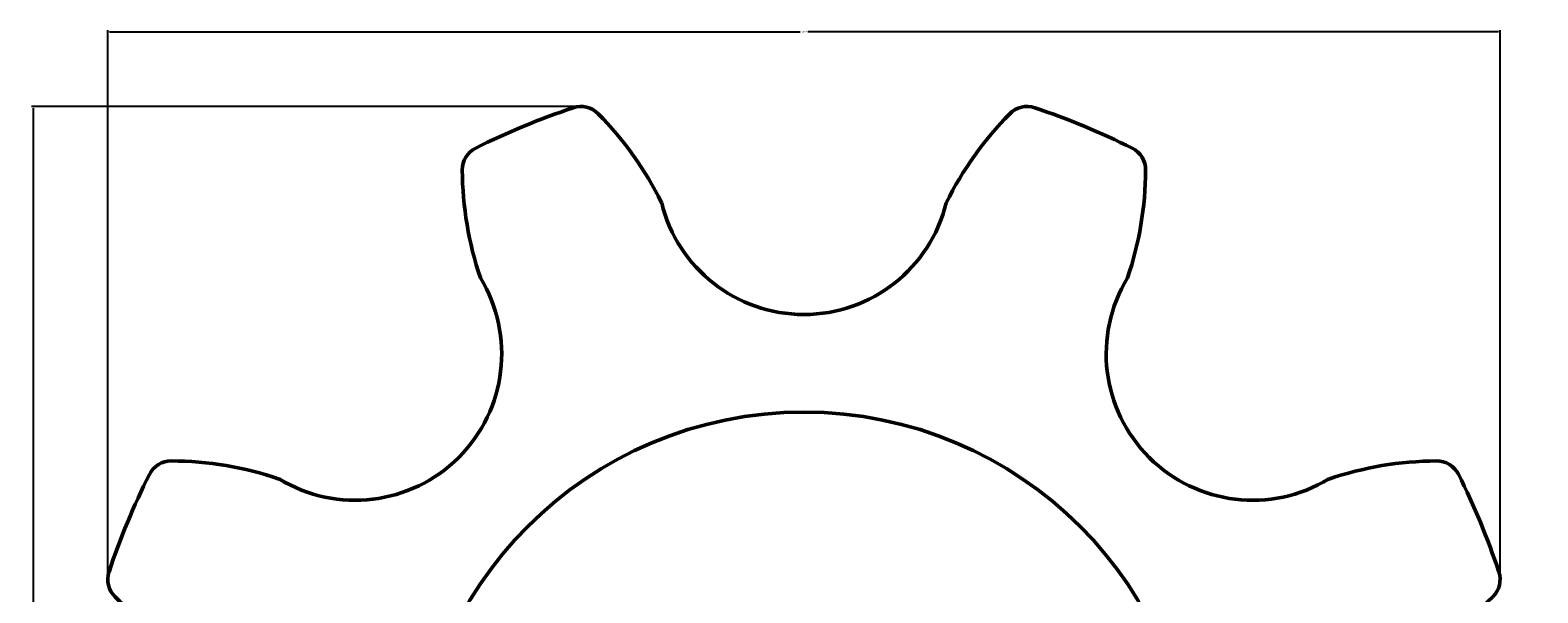
# Model space of a CAD drawing. Units: millimetres. Extents: x 7298 to 7452, y 8725 to 8883.
# Tile 2 of 2: x 7298 to 7452, y 8826 to 8883. Entities that reach past the tile are written whole.
import ezdxf

# ---------------------------------------------------------------- set-up
doc = ezdxf.new("R2010")
doc.units = ezdxf.units.MM
doc.layers.add('M-DIMS', color=2, linetype='Continuous', lineweight=18)
doc.layers.add('M-OUTL', color=7, linetype='Continuous', lineweight=50)
doc.styles.get("Standard").update_dxf_attribs({"font": 'arial.ttf'})
doc.dimstyles.get("Standard").update_dxf_attribs({"dimtxt": 0.18, "dimasz": 0.18, "dimexe": 0.18, "dimexo": 0.0625, "dimgap": 0.09, "dimtad": 0, "dimtih": 1, "dimtoh": 1, "dimdec": 4, "dimzin": 0, "dimdsep": 46, "dimtxsty": 'Standard', "dimcen": 0.09, "dimadec": 0, "dimazin": 0, "dimtfac": 1, "dimtdec": 4, "dimtofl": 0, "dimtmove": 0, "dimatfit": 3, "dimfxl": 1, "dimtolj": 1, "dimtzin": 0, "dimarcsym": 0})

# ---------------------------------------------------------------- blocks, each defined once
blk = doc.blocks.new('*U1')
for centre, radius, start, end in [((-2.28, 7.71), 2.5, 89.661, 153.3674), ((-2.47, -24.79), 35, 71.2539, 89.661), ((62.53, -24.79), 75, 153.3674, 161.6326), ((-6.28, -1.94), 2.5, 161.6326, 225.339), ((16.57, 21.18), 35, 225.339, 243.7461)]:
    blk.add_arc(centre, radius, start, end)
blk = doc.blocks.new('*U2')
at = {"layer": 'M-OUTL', "color": 0, "linetype": 'ByBlock', "lineweight": -2, "transparency": 16777216}
for p, rotation in [((7350.2, 8866.09), 315.0000000000001), ((7401.68, 8866.87), 270), ((7438.63, 8831.03), 225), ((7315.15, 8777.66), 44.99999999999996), ((7439.42, 8779.56), 180), ((7403.58, 8742.6), 134.9999999999999), ((7352.11, 8741.82), 90)]:
    blk.add_blockref('*U1', p, dxfattribs=dict(at, rotation=rotation))
blk.add_blockref('*U1', (7314.36, 8829.13), dxfattribs=at)
blk = doc.blocks.new('*D3')
at = {"layer": 'Defpoints', "color": 0, "transparency": 16777216}
for p in [(7448.2, 8883.3), (7305.59, 8827.29), (7448.2, 8827.29)]:
    blk.add_point(p, dxfattribs=at)
at = {"layer": 'M-DIMS', "color": 0, "lineweight": -2, "transparency": 16777216}
for p, q in [((7305.59, 8827.35), (7305.59, 8883.48)), ((7305.77, 8883.3), (7376.51, 8883.3)), ((7448.02, 8883.3), (7377.28, 8883.3)), ((7448.2, 8827.35), (7448.2, 8883.48))]:
    blk.add_line(p, q, dxfattribs=at)
at = {"layer": 'M-DIMS', "color": 0, "transparency": 16777216}
for points in [[(7305.77, 8883.33), (7305.77, 8883.27), (7305.59, 8883.3)], [(7448.02, 8883.33), (7448.02, 8883.27), (7448.2, 8883.3)]]:
    blk.add_solid(points, dxfattribs=at)
at = {"layer": 'M-DIMS', "color": 0, "transparency": 16777216, "insert": (7376.89, 8883.3), "char_height": 0.18, "attachment_point": 5}
blk.add_mtext('\\A1;142.6', dxfattribs=at)
blk = doc.blocks.new('*D4')
at = {"layer": 'Defpoints', "color": 0, "transparency": 16777216}
for p in [(7297.94, 8875.65), (7353.95, 8875.65), (7353.95, 8733.04)]:
    blk.add_point(p, dxfattribs=at)
at = {"layer": 'M-DIMS', "color": 0, "lineweight": -2, "transparency": 16777216}
for p, q in [((7353.88, 8875.65), (7297.76, 8875.65)), ((7297.94, 8875.47), (7297.94, 8804.53)), ((7297.94, 8733.22), (7297.94, 8804.16)), ((7353.88, 8733.04), (7297.76, 8733.04))]:
    blk.add_line(p, q, dxfattribs=at)
at = {"layer": 'M-DIMS', "color": 0, "transparency": 16777216}
for points in [[(7297.91, 8875.47), (7297.97, 8875.47), (7297.94, 8875.65)], [(7297.91, 8733.22), (7297.97, 8733.22), (7297.94, 8733.04)]]:
    blk.add_solid(points, dxfattribs=at)
at = {"layer": 'M-DIMS', "color": 0, "transparency": 16777216, "insert": (7297.94, 8804.34), "char_height": 0.18, "attachment_point": 5}
blk.add_mtext('\\A1;142.6', dxfattribs=at)

msp = doc.modelspace()

# ---------------------------------------------------------------- linework, layer by layer
at = {"layer": 'M-OUTL'}
msp.add_circle((7376.89, 8804.34), 40, dxfattribs=at)
for centre, start, end in [((7376.89, 8869.34), 193.7128, 346.2872), ((7330.93, 8850.31), 238.7128, 31.2872), ((7422.85, 8850.31), 148.7128, 301.2872)]:
    msp.add_arc(centre, 15, start, end, dxfattribs=at)

# ---------------------------------------------------------------- block references
msp.add_blockref('*U2', (0, 0), dxfattribs=at)

# ---------------------------------------------------------------- dimensions: what is measured, and where the dimension line sits
at = {"layer": 'M-DIMS'}
dim = msp.add_linear_dim(base=(7448.2, 8883.3), p1=(7305.59, 8827.29), p2=(7448.2, 8827.29), dimstyle='Standard', override={"dimdec": 1, "dimlfac": 1, "dimrnd": 0, "dimzin": 0, "dimdsep": 46, "dimlunit": 2}, dxfattribs=at)
dim.commit()
dim.dimension.update_dxf_attribs({"geometry": '*D3', "text_midpoint": (7376.89, 8883.3)})
dim = msp.add_linear_dim(base=(7297.94, 8875.65), p1=(7353.95, 8733.04), p2=(7353.95, 8875.65), angle=90, dimstyle='Standard', override={"dimdec": 1, "dimlfac": 1, "dimrnd": 0, "dimzin": 0, "dimdsep": 46, "dimlunit": 2}, dxfattribs=at)
dim.commit()
dim.dimension.update_dxf_attribs({"geometry": '*D4', "text_midpoint": (7297.94, 8804.34)})

doc.saveas('drawing.dxf')
